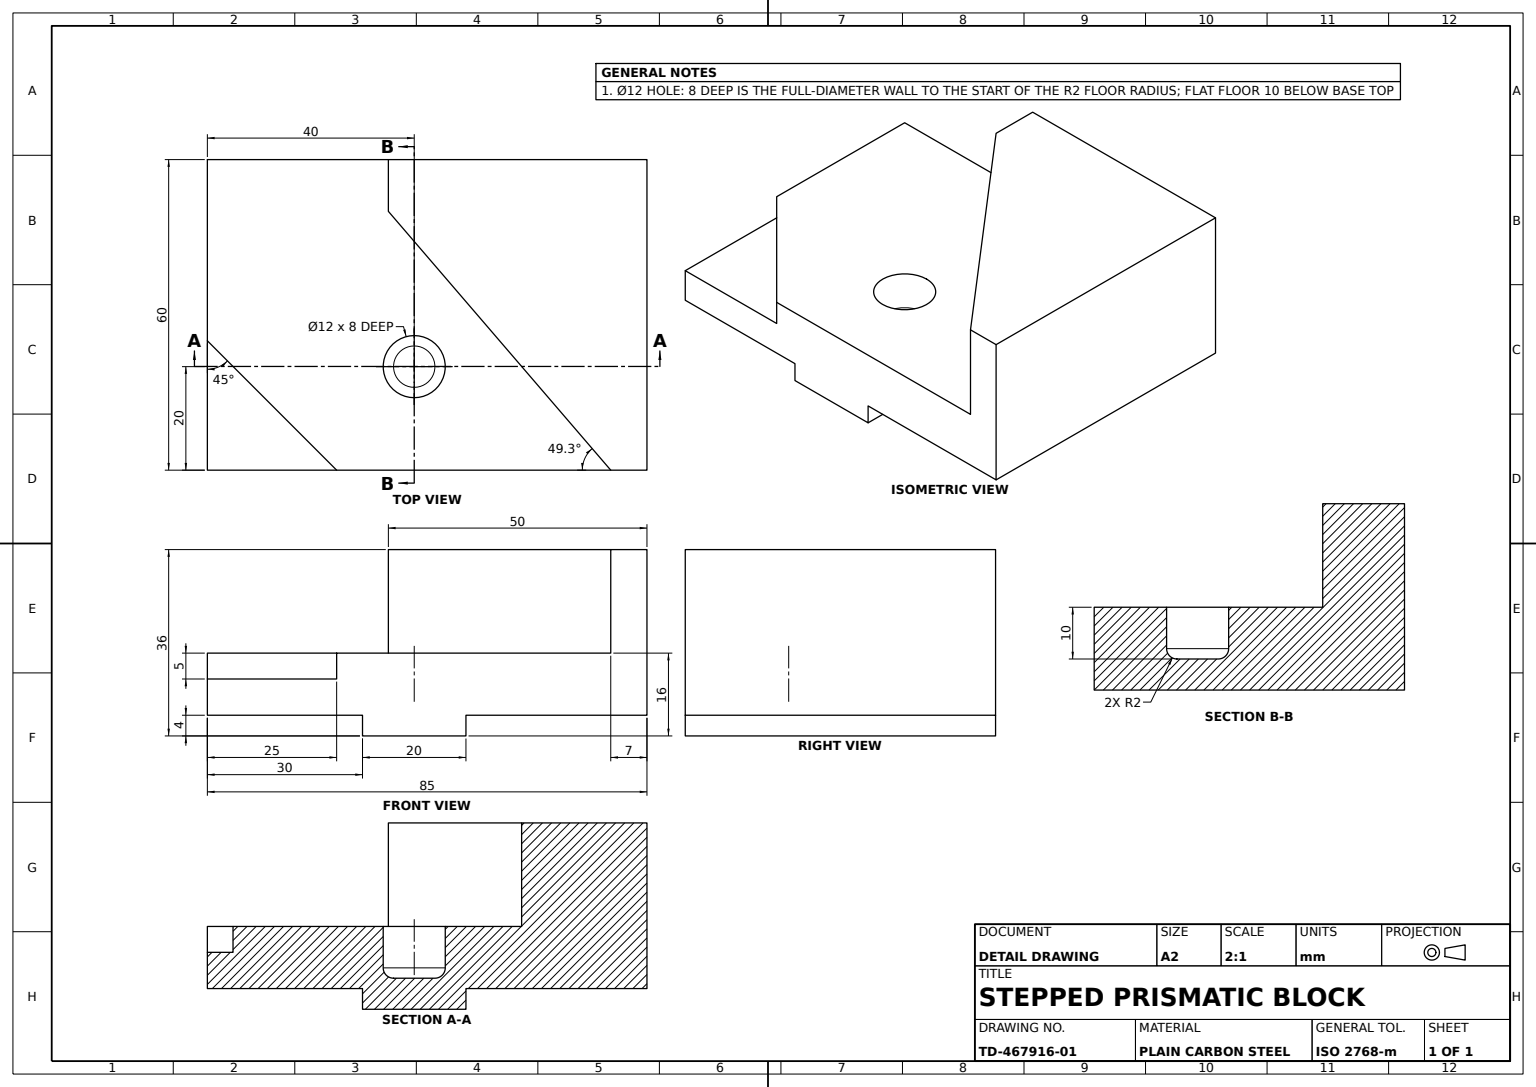
from build123d import *

# Parameters (mm, degrees)
BASE_BLOCK_SKETCH_W        = 85
BASE_BLOCK_SKETCH_H        = 60
BASE_BLOCK_85X60X16_DEPTH  = 16
UNDERSIDE_STEP_SKETCH_W    = 30
UNDERSIDE_STEP_SKETCH_H    = 4
UNDERSIDE_STEP_CUT_DEPTH   = 80.724525712
RELIEF_CUT_SKETCH_W        = 35
RELIEF_CUT_SKETCH_H        = 4
RELIEF_CUT_4MM_DEPTH       = 80.724525712
RAISED_BLOCK_20MM_DEPTH    = 20
TRIANGULAR_NOTCH_CUT_DEPTH = 5
HOLE_12_SKETCH_R           = 6
HOLE_12X10_DEPTH           = 10
FILLET_R2_R                = 2


with BuildPart() as part:
    # Base Block Sketch → Base Block 85x60x16 (new body)
    with BuildSketch(Plane(origin=(0, 0, 0), x_dir=(1, 0, 0), z_dir=(0, 1, 0))):
        with Locations((-7.5, 30)):
            Rectangle(BASE_BLOCK_SKETCH_W, BASE_BLOCK_SKETCH_H)
    extrude(amount=BASE_BLOCK_85X60X16_DEPTH)

    # Underside Step Sketch → Underside Step Cut (cut, through all)
    with BuildSketch(Plane.XY):
        with Locations((-35, 2)):
            Rectangle(UNDERSIDE_STEP_SKETCH_W, UNDERSIDE_STEP_SKETCH_H)
    extrude(amount=-UNDERSIDE_STEP_CUT_DEPTH, mode=Mode.SUBTRACT)

    # Relief Cut Sketch → Relief Cut 4mm (cut, through all)
    with BuildSketch(Plane.XY):
        with Locations((17.5, 2)):
            Rectangle(RELIEF_CUT_SKETCH_W, RELIEF_CUT_SKETCH_H)
    extrude(amount=-RELIEF_CUT_4MM_DEPTH, mode=Mode.SUBTRACT)

    # Raised Block Sketch → Raised Block 20mm (add)
    with BuildSketch(Plane(origin=(0, 16, 0), x_dir=(1, 0, 0), z_dir=(0, 1, 0))):
        Polygon((35, 60), (-15, 60), (-15, 50), (28, 0), (35, 0), align=None)
    extrude(amount=RAISED_BLOCK_20MM_DEPTH)

    # Notch Sketch → Triangular Notch Cut (cut)
    with BuildSketch(Plane(origin=(0, 16, 0), x_dir=(1, 0, 0), z_dir=(0, 1, 0))):
        Polygon((-25, 0), (-50, 25), (-50, 0), align=None)
    extrude(amount=-TRIANGULAR_NOTCH_CUT_DEPTH, mode=Mode.SUBTRACT)

    # Hole Ø12 Sketch → Hole Ø12x10 (cut)
    with BuildSketch(Plane(origin=(0, 16, 0), x_dir=(1, 0, 0), z_dir=(0, 1, 0))):
        with Locations(Location((-10, 20, 0), (0, 0, 270))):
            Circle(HOLE_12_SKETCH_R)
    extrude(amount=-HOLE_12X10_DEPTH, mode=Mode.SUBTRACT)

    # Fillet R2
    fillet_r2_edges = [part.edges().sort_by_distance(p)[0] for p in [
        (-10, 6, -26),
    ]]
    fillet(fillet_r2_edges, radius=FILLET_R2_R)


solid = part.part
